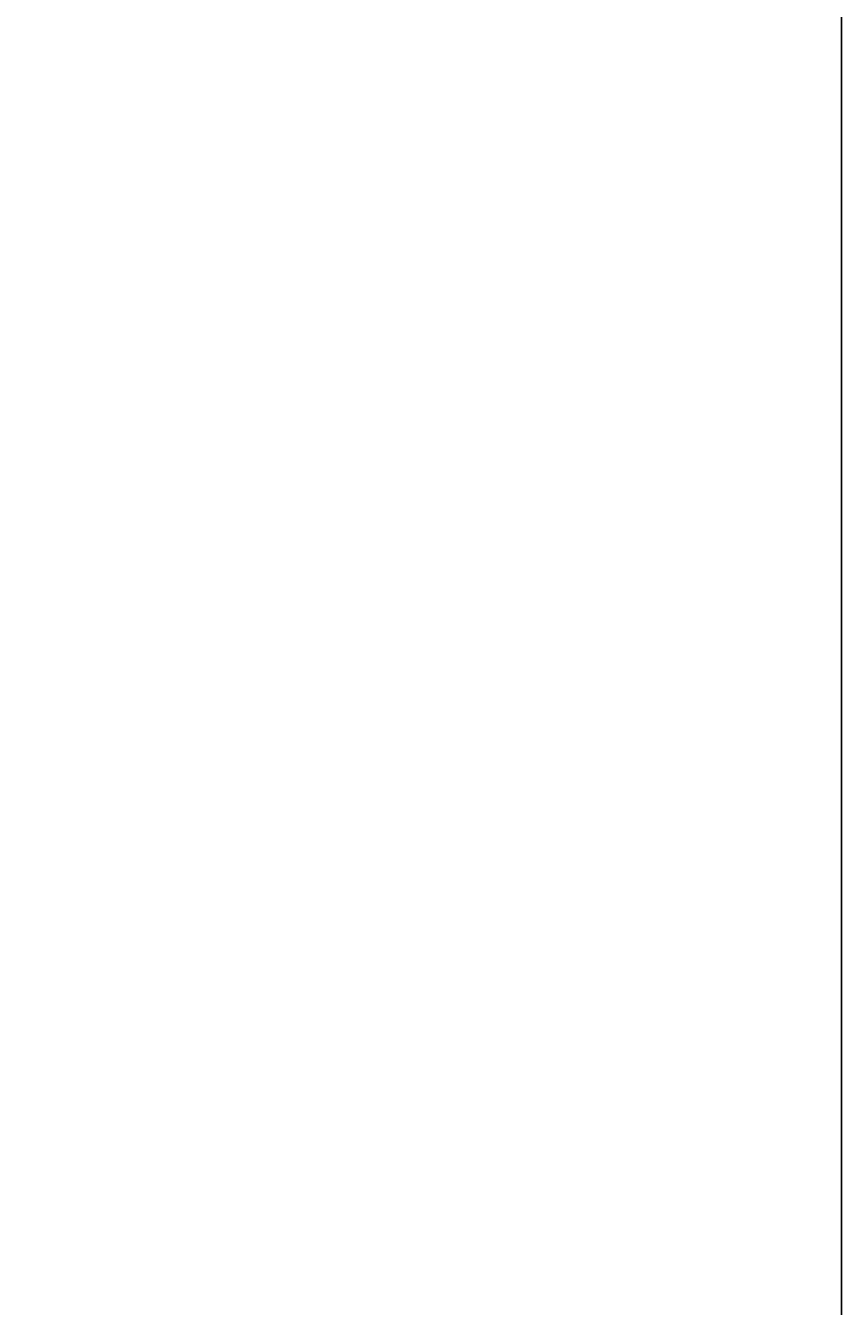
# Model space of a CAD drawing. Units: inches. Extents: x -61 to 1599, y -1316 to 257.
# Tile 29 of 204: x 365 to 404, y -851 to -790. Entities that reach past the tile are written whole.
import ezdxf

# ---------------------------------------------------------------- set-up
doc = ezdxf.new("R2010")
doc.units = ezdxf.units.IN
doc.header["$MEASUREMENT"] = 0
doc.layers.add('A-ANNO-DIMS', color=2, linetype='Continuous', lineweight=18)
doc.styles.get("Standard").update_dxf_attribs({"font": 'arial.ttf'})
doc.dimstyles.get("Standard").update_dxf_attribs({"dimtxt": 0.18, "dimasz": 0.18, "dimexe": 0.18, "dimexo": 0.0625, "dimgap": 0.09, "dimtad": 0, "dimtih": 1, "dimtoh": 1, "dimdec": 0, "dimzin": 0, "dimdsep": 46, "dimlunit": 3, "dimtxsty": 'Standard', "dimcen": 0.09, "dimadec": 0, "dimazin": 0, "dimtfac": 1, "dimtdec": 0, "dimtofl": 0, "dimtmove": 0, "dimatfit": 3, "dimfxl": 1, "dimtolj": 1, "dimtzin": 0, "dimarcsym": 0})

# ---------------------------------------------------------------- blocks, each defined once
blk = doc.blocks.new('*D710')
at = {"layer": 'A-ANNO-DIMS', "color": 0, "lineweight": -2, "transparency": 16777216}
for p, q in [((319.703, -465.385), (319.703, -1315.725)), ((403.703, -465.385), (403.703, -1315.725)), ((319.883, -1315.545), (361.484, -1315.545)), ((403.523, -1315.545), (361.921, -1315.545))]:
    blk.add_line(p, q, dxfattribs=at)
at = {"layer": 'A-ANNO-DIMS', "color": 0, "transparency": 16777216}
for points in [[(319.883, -1315.515), (319.883, -1315.575), (319.703, -1315.545)], [(403.523, -1315.515), (403.523, -1315.575), (403.703, -1315.545)]]:
    blk.add_solid(points, dxfattribs=at)
at = {"layer": 'DEFPOINTS', "color": 0, "transparency": 16777216}
for p in [(319.703, -465.323), (403.703, -465.323), (403.703, -1315.545)]:
    blk.add_point(p, dxfattribs=at)
at = {"layer": 'A-ANNO-DIMS', "color": 0, "transparency": 16777216, "insert": (361.703, -1315.545), "char_height": 0.18, "attachment_point": 5}
blk.add_mtext('\\A1;84', dxfattribs=at)

msp = doc.modelspace()

# ---------------------------------------------------------------- dimensions: what is measured, and where the dimension line sits
at = {"layer": 'A-ANNO-DIMS'}
dim = msp.add_linear_dim(base=(403.7028, -1315.5446), p1=(319.7028, -465.3229), p2=(403.7028, -465.3229), dimstyle='Standard', override={"dimdec": 0, "dimlfac": 1, "dimrnd": 0, "dimzin": 0, "dimdsep": 46, "dimlunit": 2}, dxfattribs=at)
dim.commit()
dim.dimension.update_dxf_attribs({"geometry": '*D710', "text_midpoint": (361.7028, -1315.5446)})

doc.saveas('drawing.dxf')
